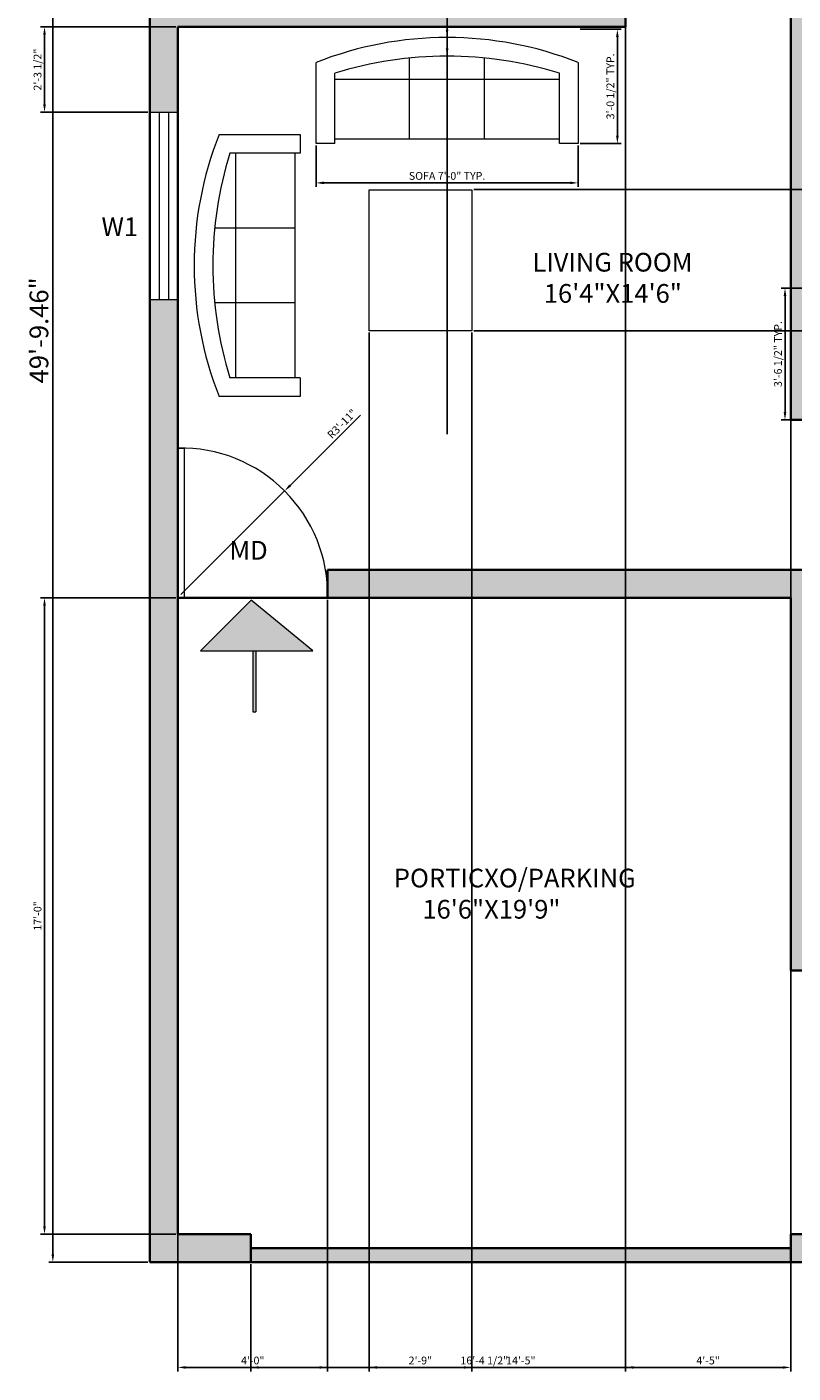
# Model space of a CAD drawing. Units: inches. Extents: x 5030 to 5465, y 5339 to 6047.
# Tile 1 of 5: x 5030 to 5275, y 5339 to 5771. Entities that reach past the tile are written whole.
import ezdxf

# ---------------------------------------------------------------- set-up
doc = ezdxf.new("R2010")
doc.units = ezdxf.units.IN
for name, color, linetype, lineweight in [('A-ANNO-DIMS', 2, 'Continuous', 18), ('A-ANNO-SYMB', 1, 'Continuous', 18), ('A-ANNO-TEXT', 7, 'Continuous', 18), ('A-AREA-IDEN', 7, 'Continuous', 25), ('A-DOOR', 3, 'Continuous', 18), ('A-FURN', 8, 'Continuous', 18), ('A-GLAZ', 4, 'Continuous', 18), ('A-WALL', 7, 'Continuous', 35)]:
    doc.layers.add(name, color=color, linetype=linetype, lineweight=lineweight)
doc.layers.add('A-WALL-PATT', color=149, linetype='Continuous', lineweight=13, true_color=0x444546)
doc.styles.get("Standard").update_dxf_attribs({"font": 'arial.ttf'})
doc.dimstyles.new('ISO-25', dxfattribs={"dimtxt": 2.5, "dimasz": 2.5, "dimexe": 1.25, "dimexo": 0.625, "dimtad": 1, "dimlunit": 3, "dimtxsty": 'Standard', "dimcen": 2.5, "dimadec": 0, "dimazin": 0, "dimtfac": 1, "dimtmove": 0, "dimatfit": 3, "dimfxl": 1, "dimarcsym": 0})

# ---------------------------------------------------------------- blocks, each defined once
blk = doc.blocks.new('Sofa - Roundback 7 ft.')
for p, q in [((-12.00002, -32.4421), (-12.00003, -6.5971)), ((11.99997, -32.4421), (11.99998, -6.5971)), ((-36.000027, -34), (-36.000027, -11.4696)), ((35.99998, -34), (35.99998, -11.4696)), ((-35.999844, -13.3819), (35.9998, -13.3819)), ((-36.000027, -32.4421), (35.99998, -32.4421))]:
    blk.add_line(p, q)
for points in [[(-36.000027, -34), (-42.000027, -34), (-42.000027, -8)], [(41.99998, -8), (41.99998, -34), (35.99998, -34)]]:
    blk.add_lwpolyline(points)
for centre, radius, start, end in [((0, -114.25), 114.25, 68.43141, 111.5686), ((-0.00001, -127.1968), 121.1968, 72.72033, 107.2797)]:
    blk.add_arc(centre, radius, start, end)
blk = doc.blocks.new('*D8')
at = {"layer": 'A-ANNO-DIMS', "color": 0, "lineweight": -2, "transparency": 16777216}
for p, q in [((5068.62, 5971.96), (5036.91, 5971.96)), ((5038.16, 5969.46), (5038.16, 5377)), ((5068.62, 5374.5), (5036.91, 5374.5))]:
    blk.add_line(p, q, dxfattribs=at)
at = {"layer": 'A-ANNO-DIMS', "color": 0, "transparency": 16777216}
for points in [[(5037.74, 5969.46), (5038.58, 5969.46), (5038.16, 5971.96)], [(5037.74, 5377), (5038.58, 5377), (5038.16, 5374.5)]]:
    blk.add_solid(points, dxfattribs=at)
at = {"layer": 'Defpoints', "color": 0, "transparency": 16777216}
for p in [(5069.24, 5971.96), (5038.16, 5374.5), (5069.24, 5374.5)]:
    blk.add_point(p, dxfattribs=at)
at = {"layer": 'A-ANNO-DIMS', "color": 0, "transparency": 16777216, "insert": (5034.47, 5673.23), "char_height": 6, "attachment_point": 5, "rotation": 90}
blk.add_mtext('49\'-9.46"', dxfattribs=at)
blk = doc.blocks.new('WIN-60IN')
for p, q in [((0, 60), (9, 60)), ((3, 60), (3, 0)), ((6, 60), (6, 0)), ((0, 0), (9, 0))]:
    blk.add_line(p, q)
blk = doc.blocks.new('*D18')
at = {"layer": 'A-ANNO-DIMS', "color": 0, "lineweight": -2, "transparency": 16777216}
for p, q in [((5278.62, 5686.78), (5271.65, 5686.78)), ((5272.9, 5647), (5272.9, 5684.28)), ((5278.62, 5644.5), (5271.65, 5644.5))]:
    blk.add_line(p, q, dxfattribs=at)
at = {"layer": 'A-ANNO-DIMS', "color": 0, "transparency": 16777216}
for points in [[(5272.48, 5684.28), (5273.32, 5684.28), (5272.9, 5686.78)], [(5272.48, 5647), (5273.32, 5647), (5272.9, 5644.5)]]:
    blk.add_solid(points, dxfattribs=at)
at = {"layer": 'Defpoints', "color": 0, "transparency": 16777216}
for p in [(5272.9, 5686.78), (5279.24, 5686.78), (5279.24, 5644.5)]:
    blk.add_point(p, dxfattribs=at)
at = {"layer": 'A-ANNO-DIMS', "color": 0, "transparency": 16777216, "insert": (5270.98, 5665.64), "char_height": 2.5, "attachment_point": 5, "rotation": 90}
blk.add_mtext('3\'-6 1/2" TYP.', dxfattribs=at)
blk = doc.blocks.new('*D19')
at = {"layer": 'A-ANNO-DIMS', "color": 0, "lineweight": -2, "transparency": 16777216}
for p, q in [((5122.56, 5732.48), (5122.56, 5719.25)), ((5206.56, 5732.48), (5206.56, 5719.25)), ((5125.06, 5720.5), (5204.06, 5720.5))]:
    blk.add_line(p, q, dxfattribs=at)
at = {"layer": 'A-ANNO-DIMS', "color": 0, "transparency": 16777216}
for points in [[(5125.06, 5720.92), (5125.06, 5720.09), (5122.56, 5720.5)], [(5204.06, 5720.92), (5204.06, 5720.09), (5206.56, 5720.5)]]:
    blk.add_solid(points, dxfattribs=at)
at = {"layer": 'Defpoints', "color": 0, "transparency": 16777216}
for p in [(5122.56, 5733.1), (5206.56, 5733.1), (5206.56, 5720.5)]:
    blk.add_point(p, dxfattribs=at)
at = {"layer": 'A-ANNO-DIMS', "color": 0, "transparency": 16777216, "insert": (5164.56, 5722.42), "char_height": 2.5, "attachment_point": 5}
blk.add_mtext('SOFA 7\'-0" TYP.', dxfattribs=at)
blk = doc.blocks.new('*D20')
at = {"layer": 'A-ANNO-DIMS', "color": 0, "lineweight": -2, "transparency": 16777216}
for p, q in [((5207.18, 5769.77), (5220.41, 5769.77)), ((5219.16, 5735.6), (5219.16, 5767.27)), ((5207.18, 5733.1), (5220.41, 5733.1))]:
    blk.add_line(p, q, dxfattribs=at)
at = {"layer": 'A-ANNO-DIMS', "color": 0, "transparency": 16777216}
for points in [[(5218.74, 5767.27), (5219.58, 5767.27), (5219.16, 5769.77)], [(5218.74, 5735.6), (5219.58, 5735.6), (5219.16, 5733.1)]]:
    blk.add_solid(points, dxfattribs=at)
at = {"layer": 'Defpoints', "color": 0, "transparency": 16777216}
for p in [(5206.56, 5769.77), (5219.16, 5769.77), (5206.56, 5733.1)]:
    blk.add_point(p, dxfattribs=at)
at = {"layer": 'A-ANNO-DIMS', "color": 0, "transparency": 16777216, "insert": (5217.24, 5751.44), "char_height": 2.5, "attachment_point": 5, "rotation": 90}
blk.add_mtext('3\'-0 1/2" TYP.', dxfattribs=at)
blk = doc.blocks.new('*D33')
at = {"layer": 'A-ANNO-DIMS', "color": 0, "lineweight": -2, "transparency": 16777216}
for p, q in [((5078.24, 5586.88), (5078.24, 5339.5)), ((5126.24, 5586.88), (5126.24, 5339.5)), ((5080.74, 5340.75), (5123.74, 5340.75))]:
    blk.add_line(p, q, dxfattribs=at)
at = {"layer": 'A-ANNO-DIMS', "color": 0, "transparency": 16777216}
for points in [[(5080.74, 5341.17), (5080.74, 5340.34), (5078.24, 5340.75)], [(5123.74, 5341.17), (5123.74, 5340.34), (5126.24, 5340.75)]]:
    blk.add_solid(points, dxfattribs=at)
at = {"layer": 'Defpoints', "color": 0, "transparency": 16777216}
for p in [(5078.24, 5587.5), (5126.24, 5587.5), (5126.24, 5340.75)]:
    blk.add_point(p, dxfattribs=at)
at = {"layer": 'A-ANNO-DIMS', "color": 0, "transparency": 16777216, "insert": (5102.24, 5342.65), "char_height": 2.5, "attachment_point": 5}
blk.add_mtext('4\'-0"', dxfattribs=at)
blk = doc.blocks.new('*D34')
at = {"layer": 'A-ANNO-DIMS', "color": 0, "lineweight": -2, "transparency": 16777216}
for p, q in [((5078.24, 5382.88), (5078.24, 5339.5)), ((5274.74, 5382.88), (5274.74, 5339.5)), ((5080.74, 5340.75), (5272.24, 5340.75))]:
    blk.add_line(p, q, dxfattribs=at)
at = {"layer": 'A-ANNO-DIMS', "color": 0, "transparency": 16777216}
for points in [[(5080.74, 5341.17), (5080.74, 5340.34), (5078.24, 5340.75)], [(5272.24, 5341.17), (5272.24, 5340.34), (5274.74, 5340.75)]]:
    blk.add_solid(points, dxfattribs=at)
at = {"layer": 'Defpoints', "color": 0, "transparency": 16777216}
for p in [(5078.24, 5383.5), (5274.74, 5383.5), (5274.74, 5340.75)]:
    blk.add_point(p, dxfattribs=at)
at = {"layer": 'A-ANNO-DIMS', "color": 0, "transparency": 16777216, "insert": (5176.49, 5342.67), "char_height": 2.5, "attachment_point": 5}
blk.add_mtext('16\'-4 1/2"', dxfattribs=at)
blk = doc.blocks.new('*D35')
at = {"layer": 'A-ANNO-DIMS', "color": 0, "lineweight": -2, "transparency": 16777216}
for p, q in [((5077.62, 5587.5), (5034.24, 5587.5)), ((5035.49, 5386), (5035.49, 5585)), ((5077.62, 5383.5), (5034.24, 5383.5))]:
    blk.add_line(p, q, dxfattribs=at)
at = {"layer": 'A-ANNO-DIMS', "color": 0, "transparency": 16777216}
for points in [[(5035.07, 5585), (5035.91, 5585), (5035.49, 5587.5)], [(5035.07, 5386), (5035.91, 5386), (5035.49, 5383.5)]]:
    blk.add_solid(points, dxfattribs=at)
at = {"layer": 'Defpoints', "color": 0, "transparency": 16777216}
for p in [(5035.49, 5587.5), (5078.24, 5587.5), (5078.24, 5383.5)]:
    blk.add_point(p, dxfattribs=at)
at = {"layer": 'A-ANNO-DIMS', "color": 0, "transparency": 16777216, "insert": (5033.59, 5485.5), "char_height": 2.5, "attachment_point": 5, "rotation": 90}
blk.add_mtext('17\'-0"', dxfattribs=at)
blk = doc.blocks.new('*D48')
at = {"layer": 'A-ANNO-DIMS', "color": 0, "lineweight": -2, "transparency": 16777216}
for p, q in [((5077.62, 5770.5), (5034.24, 5770.5)), ((5035.49, 5745.65), (5035.49, 5768)), ((5068.62, 5743.15), (5034.24, 5743.15))]:
    blk.add_line(p, q, dxfattribs=at)
at = {"layer": 'A-ANNO-DIMS', "color": 0, "transparency": 16777216}
for points in [[(5035.07, 5768), (5035.91, 5768), (5035.49, 5770.5)], [(5035.07, 5745.65), (5035.91, 5745.65), (5035.49, 5743.15)]]:
    blk.add_solid(points, dxfattribs=at)
at = {"layer": 'Defpoints', "color": 0, "transparency": 16777216}
for p in [(5035.49, 5770.5), (5078.24, 5770.5), (5069.24, 5743.15)]:
    blk.add_point(p, dxfattribs=at)
at = {"layer": 'A-ANNO-DIMS', "color": 0, "transparency": 16777216, "insert": (5033.57, 5756.83), "char_height": 2.5, "attachment_point": 5, "rotation": 90}
blk.add_mtext('2\'-3 1/2"', dxfattribs=at)
blk = doc.blocks.new('*D55')
at = {"layer": 'A-ANNO-DIMS', "color": 0, "lineweight": -2, "transparency": 16777216}
for p, q in [((5221.75, 5774.38), (5221.75, 5339.5)), ((5274.74, 5774.38), (5274.74, 5339.5)), ((5224.25, 5340.75), (5272.24, 5340.75))]:
    blk.add_line(p, q, dxfattribs=at)
at = {"layer": 'A-ANNO-DIMS', "color": 0, "transparency": 16777216}
for points in [[(5224.25, 5341.17), (5224.25, 5340.34), (5221.75, 5340.75)], [(5272.24, 5341.17), (5272.24, 5340.34), (5274.74, 5340.75)]]:
    blk.add_solid(points, dxfattribs=at)
at = {"layer": 'Defpoints', "color": 0, "transparency": 16777216}
for p in [(5221.75, 5775), (5274.74, 5775), (5274.74, 5340.75)]:
    blk.add_point(p, dxfattribs=at)
at = {"layer": 'A-ANNO-DIMS', "color": 0, "transparency": 16777216, "insert": (5248.24, 5342.65), "char_height": 2.5, "attachment_point": 5}
blk.add_mtext('4\'-5"', dxfattribs=at)
blk = doc.blocks.new('*D58')
at = {"layer": 'A-ANNO-DIMS', "color": 0, "lineweight": -2, "transparency": 16777216}
for p, q in [((5139.55, 5672.49), (5139.55, 5339.5)), ((5172.45, 5672.49), (5172.45, 5339.5)), ((5142.05, 5340.75), (5169.95, 5340.75))]:
    blk.add_line(p, q, dxfattribs=at)
at = {"layer": 'A-ANNO-DIMS', "color": 0, "transparency": 16777216}
for points in [[(5142.05, 5341.17), (5142.05, 5340.34), (5139.55, 5340.75)], [(5169.95, 5341.17), (5169.95, 5340.34), (5172.45, 5340.75)]]:
    blk.add_solid(points, dxfattribs=at)
at = {"layer": 'Defpoints', "color": 0, "transparency": 16777216}
for p in [(5139.55, 5673.12), (5172.45, 5673.12), (5172.45, 5340.75)]:
    blk.add_point(p, dxfattribs=at)
at = {"layer": 'A-ANNO-DIMS', "color": 0, "transparency": 16777216, "insert": (5156, 5342.65), "char_height": 2.5, "attachment_point": 5}
blk.add_mtext('2\'-9"', dxfattribs=at)
blk = doc.blocks.new('*D59')
at = {"layer": 'A-ANNO-DIMS', "color": 0, "lineweight": -2, "transparency": 16777216}
for p, q in [((5173.08, 5718.33), (5464.24, 5718.33)), ((5462.99, 5675.62), (5462.99, 5715.83)), ((5173.08, 5673.12), (5464.24, 5673.12))]:
    blk.add_line(p, q, dxfattribs=at)
at = {"layer": 'A-ANNO-DIMS', "color": 0, "transparency": 16777216}
for points in [[(5462.57, 5715.83), (5463.41, 5715.83), (5462.99, 5718.33)], [(5462.57, 5675.62), (5463.41, 5675.62), (5462.99, 5673.12)]]:
    blk.add_solid(points, dxfattribs=at)
at = {"layer": 'Defpoints', "color": 0, "transparency": 16777216}
for p in [(5172.45, 5718.33), (5462.99, 5718.33), (5172.45, 5673.12)]:
    blk.add_point(p, dxfattribs=at)
at = {"layer": 'A-ANNO-DIMS', "color": 0, "transparency": 16777216, "insert": (5461.09, 5695.72), "char_height": 2.5, "attachment_point": 5, "rotation": 90}
blk.add_mtext('3\'-9"', dxfattribs=at)
blk = doc.blocks.new('*D60')
at = {"layer": 'A-ANNO-DIMS', "color": 0, "lineweight": -2, "transparency": 16777216}
for p, q in [((5101.67, 5373.88), (5101.67, 5339.5)), ((5274.74, 5373.88), (5274.74, 5339.5)), ((5104.17, 5340.75), (5272.24, 5340.75))]:
    blk.add_line(p, q, dxfattribs=at)
at = {"layer": 'A-ANNO-DIMS', "color": 0, "transparency": 16777216}
for points in [[(5104.17, 5341.17), (5104.17, 5340.34), (5101.67, 5340.75)], [(5272.24, 5341.17), (5272.24, 5340.34), (5274.74, 5340.75)]]:
    blk.add_solid(points, dxfattribs=at)
at = {"layer": 'Defpoints', "color": 0, "transparency": 16777216}
for p in [(5101.67, 5374.5), (5274.74, 5374.5), (5274.74, 5340.75)]:
    blk.add_point(p, dxfattribs=at)
at = {"layer": 'A-ANNO-DIMS', "color": 0, "transparency": 16777216, "insert": (5188.2, 5342.65), "char_height": 2.5, "attachment_point": 5}
blk.add_mtext('14\'-5"', dxfattribs=at)
blk = doc.blocks.new('*D63')
at = {"layer": 'A-ANNO-DIMS', "color": 0, "lineweight": -2, "transparency": 16777216}
for p, q in [((5136.75, 5646.01), (5114.25, 5623.51)), ((5079.24, 5588.5), (5112.48, 5621.74))]:
    blk.add_line(p, q, dxfattribs=at)
at = {"layer": 'A-ANNO-DIMS', "color": 0, "transparency": 16777216}
blk.add_solid([(5113.95, 5623.81), (5114.54, 5623.22), (5112.48, 5621.74)], dxfattribs=at)
at = {"layer": 'Defpoints', "color": 0, "transparency": 16777216}
for p in [(5112.48, 5621.74), (5079.24, 5588.5)]:
    blk.add_point(p, dxfattribs=at)
at = {"layer": 'A-ANNO-DIMS', "color": 0, "transparency": 16777216, "insert": (5131.08, 5643.03), "char_height": 2.5, "attachment_point": 5, "rotation": 45.0001}
blk.add_mtext('R3\'-11"', dxfattribs=at)
blk = doc.blocks.new('*D66')
at = {"layer": 'A-ANNO-DIMS', "color": 0, "lineweight": -2, "transparency": 16777216}
for p, q in [((5164.56, 5842.64), (5164.56, 5763.6)), ((5164.56, 5639.91), (5164.56, 5761.1))]:
    blk.add_line(p, q, dxfattribs=at)
at = {"layer": 'A-ANNO-DIMS', "color": 0, "transparency": 16777216}
blk.add_solid([(5164.14, 5763.6), (5164.98, 5763.6), (5164.56, 5761.1)], dxfattribs=at)
at = {"layer": 'Defpoints', "color": 0, "transparency": 16777216}
for p in [(5164.56, 5761.1), (5164.56, 5639.91)]:
    blk.add_point(p, dxfattribs=at)
at = {"layer": 'A-ANNO-DIMS', "color": 0, "transparency": 16777216, "insert": (5162.66, 5833.82), "char_height": 2.5, "attachment_point": 5, "rotation": 89.9998}
blk.add_mtext('2X R10\'-1"', dxfattribs=at)
blk = doc.blocks.new('*D67')
at = {"layer": 'A-ANNO-DIMS', "color": 0, "lineweight": -2, "transparency": 16777216}
for p, q in [((5164.56, 5846.42), (5164.56, 5769.6)), ((5164.56, 5652.85), (5164.56, 5767.1))]:
    blk.add_line(p, q, dxfattribs=at)
at = {"layer": 'A-ANNO-DIMS', "color": 0, "transparency": 16777216}
blk.add_solid([(5164.14, 5769.6), (5164.98, 5769.6), (5164.56, 5767.1)], dxfattribs=at)
at = {"layer": 'Defpoints', "color": 0, "transparency": 16777216}
for p in [(5164.56, 5767.1), (5164.56, 5652.85)]:
    blk.add_point(p, dxfattribs=at)
at = {"layer": 'A-ANNO-DIMS', "color": 0, "transparency": 16777216, "insert": (5162.64, 5835.65), "char_height": 2.5, "attachment_point": 5, "rotation": 89.9998}
blk.add_mtext('2X R9\'-6 1/2"', dxfattribs=at)

msp = doc.modelspace()

# ---------------------------------------------------------------- hatches: boundary and pattern name
at = {"layer": 'A-ANNO-SYMB'}
h = msp.add_hatch(color=256, dxfattribs=at)
h.dxf.hatch_style = 1
h.paths.add_polyline_path([(5101.785, 5586.691), (5085.517, 5570.533), (5089.992, 5570.533), (5121.542, 5570.533)])
h.paths.add_polyline_path([(5103.291, 5570.533), (5102.291, 5570.533), (5102.291, 5550.944), (5103.291, 5550.944)])
at = {"layer": 'A-WALL-PATT'}
h = msp.add_hatch(color=256, dxfattribs=at)
h.dxf.hatch_style = 1
h.paths.add_polyline_path([(5227.999, 5974.503), (5069.24, 5974.503), (5069.24, 5942.38), (5078.24, 5942.38), (5078.24, 5965.503), (5198.24, 5965.503), (5198.24, 5916.003), (5274.74, 5916.003), (5274.74, 5869.503), (5202.74, 5869.503), (5202.74, 5898.003), (5198.24, 5898.003), (5198.24, 5865.003), (5274.74, 5865.003), (5274.74, 5817.003, -0.0121933), (5276.74, 5817.003), (5279.24, 5817.003), (5279.24, 5947.503, -0.0293864), (5277.24, 5947.503), (5274.74, 5947.503), (5274.74, 5920.503), (5202.74, 5920.503), (5202.74, 5965.503), (5227.999, 5965.503)])
h.paths.add_polyline_path([(5078.24, 5894.38), (5069.24, 5894.38), (5069.24, 5845.837), (5078.24, 5845.837), (5078.24, 5865.003), (5138.24, 5865.003), (5138.24, 5869.503), (5078.24, 5869.503)], flags=17)
h.paths.add_polyline_path([(5316.341, 5974.503), (5251.999, 5974.503), (5251.999, 5965.503), (5279.24, 5965.503), (5316.341, 5965.503)])
h.paths.add_polyline_path([(5429.24, 5974.503), (5376.341, 5974.503), (5376.341, 5965.503), (5420.24, 5965.503), (5420.24, 5904.986), (5429.24, 5904.986)])
h.paths.add_polyline_path([(5429.24, 5844.986), (5420.24, 5844.986), (5420.24, 5773.503), (5279.24, 5773.503), (5279.24, 5775.003), (5274.74, 5775.003), (5274.74, 5644.503), (5279.24, 5644.503), (5279.24, 5686.503), (5279.24, 5769.003), (5420.24, 5769.003), (5420.24, 5738.095), (5429.24, 5738.095)])
h.paths.add_polyline_path([(5429.24, 5678.095), (5420.24, 5678.095), (5420.24, 5649.003), (5321.24, 5649.003), (5321.24, 5646.503, -0.0121933), (5321.24, 5644.503), (5343.74, 5644.503), (5343.74, 5614.503, -0.0293864), (5345.74, 5614.503), (5348.24, 5614.503), (5348.24, 5644.503), (5420.24, 5644.503), (5420.24, 5636.807), (5429.24, 5636.807)])
h.paths.add_polyline_path([(5429.24, 5612.807), (5420.24, 5612.807), (5420.24, 5596.503), (5321.24, 5596.503, -0.0121933), (5321.24, 5594.503), (5321.24, 5592.003), (5420.24, 5592.003), (5420.24, 5566.431), (5429.24, 5566.431)])
h.paths.add_polyline_path([(5429.24, 5506.431), (5420.24, 5506.431), (5420.24, 5472.003), (5279.24, 5472.003), (5279.24, 5596.503), (5126.24, 5596.503), (5126.24, 5589.503, -0.0106371), (5126.24, 5587.503), (5274.74, 5587.503), (5274.74, 5468.003), (5420.24, 5468.003), (5420.24, 5452.536), (5429.24, 5452.536)])
h.paths.add_polyline_path([(5429.24, 5392.536), (5420.24, 5392.536), (5420.24, 5383.503), (5274.74, 5383.503), (5274.74, 5374.503), (5429.24, 5374.503)])
h.paths.add_polyline_path([(5101.667, 5383.503), (5078.24, 5383.503), (5078.24, 5683.152), (5069.24, 5683.152), (5069.24, 5374.503), (5101.667, 5374.503)])
h.paths.add_polyline_path([(5078.24, 5770.503), (5221.745, 5770.503), (5221.745, 5775.003), (5078.24, 5775.003), (5078.24, 5785.837), (5069.24, 5785.837), (5069.24, 5743.152), (5078.24, 5743.152)])
h.paths.add_polyline_path([(5274.74, 5379.003), (5101.667, 5379.003), (5101.667, 5374.503), (5274.74, 5374.503)])

# ---------------------------------------------------------------- linework, layer by layer
at = {"layer": 'A-ANNO-SYMB'}
for p, q in [((5101.785, 5586.691), (5085.517, 5570.533)), ((5121.542, 5570.533), (5101.785, 5586.691)), ((5085.517, 5570.533), (5089.992, 5570.533)), ((5089.992, 5570.533), (5121.542, 5570.533)), ((5102.291, 5570.533), (5102.291, 5550.944)), ((5103.291, 5570.533), (5103.291, 5550.944)), ((5121.542, 5570.533), (5121.542, 5570.533)), ((5102.291, 5550.944), (5103.291, 5550.944))]:
    msp.add_line(p, q, dxfattribs=at)
at = {"layer": 'A-DOOR'}
for p, q in [((5078.24, 5587.503), (5078.24, 5635.503)), ((5078.24, 5635.503), (5080.24, 5635.503)), ((5080.24, 5635.503), (5080.24, 5587.503)), ((5080.24, 5587.503), (5078.24, 5587.503))]:
    msp.add_line(p, q, dxfattribs=at)
msp.add_arc((5079.24, 5588.503), 47.011, 358.78112, 91.21888, dxfattribs=at)
at = {"layer": 'A-FURN'}
msp.add_lwpolyline([(5139.546, 5718.328), (5172.454, 5718.328), (5172.454, 5673.117), (5139.546, 5673.117)], close=True, dxfattribs=at)
at = {"layer": 'A-WALL'}
for p, q in [((5069.24, 5374.503), (5069.24, 5974.503)), ((5221.745, 5775.003), (5221.745, 5770.503)), ((5274.74, 5644.503), (5274.74, 5775.003)), ((5078.24, 5383.503), (5078.24, 5770.503)), ((5078.24, 5770.503), (5221.745, 5770.503)), ((5279.24, 5644.503), (5274.74, 5644.503)), ((5279.24, 5596.503), (5126.24, 5596.503)), ((5126.24, 5587.503), (5126.24, 5596.503)), ((5274.74, 5587.503), (5078.24, 5587.503)), ((5274.74, 5468.003), (5274.74, 5587.503)), ((5274.74, 5468.003), (5420.24, 5468.003)), ((5101.667, 5383.503), (5078.24, 5383.503)), ((5101.667, 5383.503), (5101.667, 5374.503)), ((5420.24, 5383.503), (5274.74, 5383.503)), ((5274.74, 5383.503), (5274.74, 5374.503)), ((5101.667, 5379.003), (5274.74, 5379.003)), ((5429.24, 5374.503), (5069.24, 5374.503))]:
    msp.add_line(p, q, dxfattribs=at)

# ---------------------------------------------------------------- block references
at = {"layer": 'A-FURN'}
msp.add_blockref('Sofa - Roundback 7 ft.', (5164.559, 5767.102), dxfattribs=at)
at = {"layer": 'A-FURN', "rotation": 90}
msp.add_blockref('Sofa - Roundback 7 ft.', (5083.455, 5694.033), dxfattribs=at)
at = {"layer": 'A-GLAZ'}
msp.add_blockref('WIN-60IN', (5069.24, 5683.153), dxfattribs=at)

# ---------------------------------------------------------------- texts
at = {"layer": 'A-ANNO-TEXT', "char_height": 6, "attachment_point": 1}
for s, insert in [('W1 ', (5053.75, 5709.439)), ('MD', (5094.775, 5605.719))]:
    msp.add_mtext_dynamic_manual_height_columns(s, width=54.21026, gutter_width=12.5, heights=[0], dxfattribs=dict(at, insert=insert))
at = {"layer": 'A-AREA-IDEN', "char_height": 6, "attachment_point": 1}
for s, width, heights, insert in [(' LIVING ROOM\\P   16\'4"X14\'6"', 70.66998, [42.499], (5190.079, 5698.07)), (' {\\fTimes New Roman|b0|i0|c0|p18; PORTICXO/PARKING\\P     16\'6"X19\'9"}', 75.97814, [52.555], (5147.482, 5500.641))]:
    msp.add_mtext_dynamic_manual_height_columns(s, width=width, gutter_width=12.5, heights=heights, dxfattribs=dict(at, insert=insert))

# ---------------------------------------------------------------- dimensions: what is measured, and where the dimension line sits
at = {"layer": 'A-ANNO-DIMS'}
for base, p1, p2, override, picture, middle in [((5038.161, 5374.503), (5069.24, 5971.965), (5069.24, 5374.503), {"dimtxt": 6, "dimclrd": 0, "dimclre": 0, "dimclrt": 0}, '*D8', (5034.472, 5673.234)), ((5035.49, 5770.503), (5069.24, 5743.152), (5078.24, 5770.503), {"dimdec": 1, "dimlfac": 1, "dimrnd": 0, "dimzin": 1, "dimdsep": 46, "dimlunit": 4, "dimfrac": 2}, '*D48', (5033.572, 5756.828)), ((5462.99, 5718.328), (5172.454, 5673.117), (5172.454, 5718.328), {"dimdec": 1, "dimlfac": 1, "dimrnd": 0, "dimzin": 1, "dimdsep": 46, "dimlunit": 4, "dimfrac": 2}, '*D59', (5461.088, 5695.723)), ((5035.49, 5587.503), (5078.24, 5383.503), (5078.24, 5587.503), {"dimdec": 1, "dimlfac": 1, "dimrnd": 0, "dimzin": 1, "dimdsep": 46, "dimlunit": 4, "dimfrac": 2}, '*D35', (5033.589, 5485.503))]:
    dim = msp.add_linear_dim(base=base, p1=p1, p2=p2, angle=90, dimstyle='ISO-25', override=override, dxfattribs=at)
    dim.commit()
    dim.dimension.update_dxf_attribs({"geometry": picture, "text_midpoint": middle})
for center, mpoint, picture, middle in [((5164.55865, 5652.852134), (5164.559, 5767.102134), '*D67', (5164.55921, 5835.652134)), ((5164.559, 5639.905), (5164.559, 5761.102), '*D66', (5164.559, 5833.82))]:
    dim = msp.add_radius_dim(center=center, mpoint=mpoint, text='2X <>', dimstyle='ISO-25', override={"dimdec": 1, "dimlfac": 1, "dimrnd": 0, "dimzin": 1, "dimdsep": 46, "dimlunit": 4, "dimfrac": 2}, dxfattribs=at)
    dim.commit()
    dim.dimension.update_dxf_attribs({"geometry": picture, "text_midpoint": middle, "dimtype": 164})
for base, p1, p2, picture, middle in [((5274.74, 5340.753), (5221.745, 5775.003), (5274.74, 5775.003), '*D55', (5248.243, 5342.649)), ((5172.454, 5340.753), (5139.546, 5673.117), (5172.454, 5673.117), '*D58', (5156, 5342.655)), ((5126.24, 5340.753), (5078.24, 5587.503), (5126.24, 5587.503), '*D33', (5102.24, 5342.655)), ((5274.74, 5340.753), (5078.24, 5383.503), (5274.74, 5383.503), '*D34', (5176.49, 5342.671)), ((5274.74, 5340.753), (5101.667, 5374.503), (5274.74, 5374.503), '*D60', (5188.204, 5342.655))]:
    dim = msp.add_linear_dim(base=base, p1=p1, p2=p2, dimstyle='ISO-25', override={"dimdec": 1, "dimlfac": 1, "dimrnd": 0, "dimzin": 1, "dimdsep": 46, "dimlunit": 4, "dimfrac": 2}, dxfattribs=at)
    dim.commit()
    dim.dimension.update_dxf_attribs({"geometry": picture, "text_midpoint": middle})
for base, p1, p2, picture, middle in [((5219.159, 5769.769), (5206.559, 5733.102), (5206.559, 5769.769), '*D20', (5217.24, 5751.435)), ((5272.899, 5686.777), (5279.24, 5644.503), (5279.24, 5686.777), '*D18', (5270.981, 5665.64))]:
    dim = msp.add_linear_dim(base=base, p1=p1, p2=p2, angle=90, text='<> TYP.', dimstyle='ISO-25', override={"dimdec": 1, "dimlfac": 1, "dimrnd": 0, "dimzin": 1, "dimdsep": 46, "dimlunit": 4, "dimfrac": 2}, dxfattribs=at)
    dim.commit()
    dim.dimension.update_dxf_attribs({"geometry": picture, "text_midpoint": middle})
dim = msp.add_linear_dim(base=(5206.559, 5720.502), p1=(5122.559, 5733.102), p2=(5206.559, 5733.102), text='SOFA <> TYP.', dimstyle='ISO-25', override={"dimdec": 1, "dimlfac": 1, "dimrnd": 0, "dimzin": 1, "dimdsep": 46, "dimlunit": 4, "dimfrac": 2}, dxfattribs=at)
dim.commit()
dim.dimension.update_dxf_attribs({"geometry": '*D19', "text_midpoint": (5164.559, 5722.421)})
dim = msp.add_radius_dim(center=(5079.24, 5588.503), mpoint=(5112.482, 5621.745), dimstyle='ISO-25', override={"dimdec": 1, "dimlfac": 1, "dimrnd": 0, "dimzin": 1, "dimdsep": 46, "dimlunit": 4, "dimfrac": 2}, dxfattribs=at)
dim.commit()
dim.dimension.update_dxf_attribs({"geometry": '*D63', "text_midpoint": (5132.427, 5641.69), "dimtype": 164})

doc.saveas('drawing.dxf')
